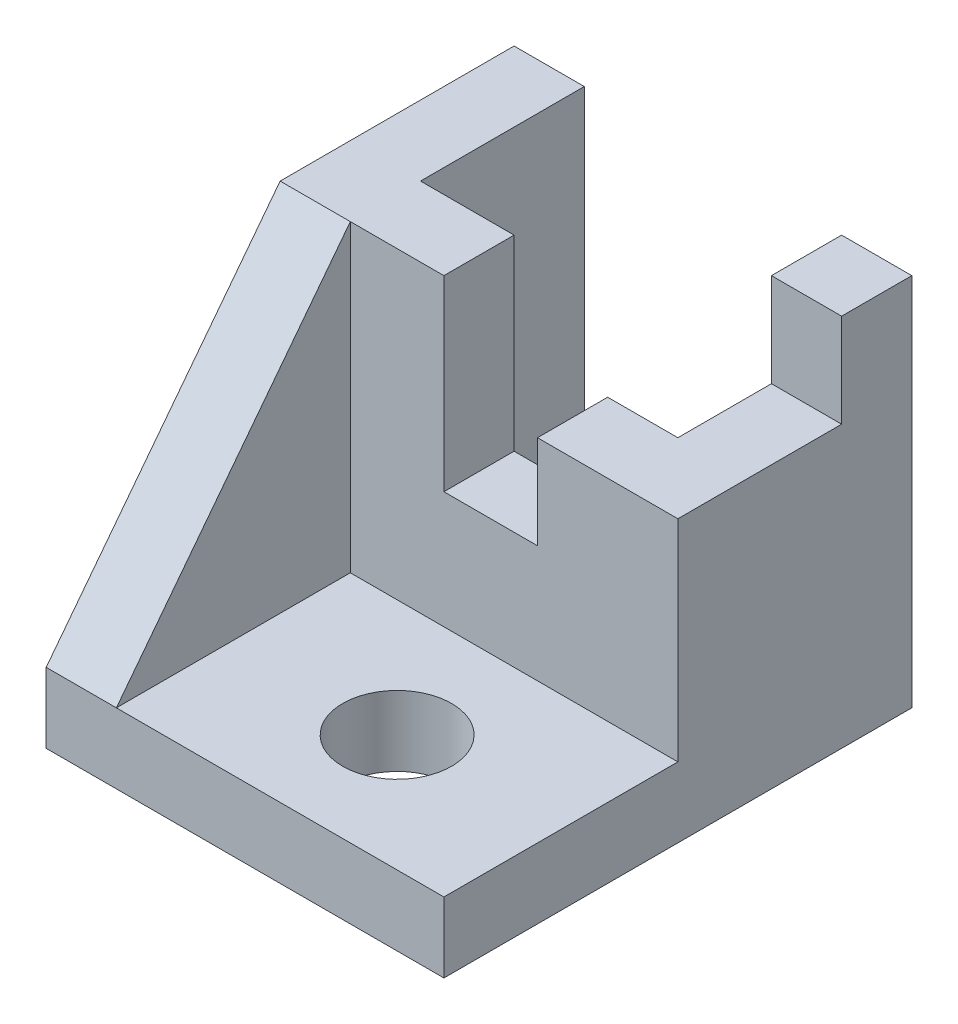
ISO-10303-21;
HEADER;
FILE_DESCRIPTION(('STEP AP214'),'2;1');
FILE_NAME('part.step','',(''),(''),'','','');
FILE_SCHEMA(('AUTOMOTIVE_DESIGN { 1 0 10303 214 1 1 1 1 }'));
ENDSEC;
DATA;
#1=APPLICATION_CONTEXT('core data for automotive mechanical design processes');
#2=APPLICATION_PROTOCOL_DEFINITION('international standard','automotive_design',2000,#1);
#3=PRODUCT_CONTEXT('',#1,'mechanical');
#4=PRODUCT('Part','Part','',(#3));
#5=PRODUCT_RELATED_PRODUCT_CATEGORY('part','',(#4));
#6=PRODUCT_DEFINITION_FORMATION('','',#4);
#7=PRODUCT_DEFINITION_CONTEXT('part definition',#1,'design');
#8=PRODUCT_DEFINITION('design','',#6,#7);
#9=PRODUCT_DEFINITION_SHAPE('','',#8);
#10=(LENGTH_UNIT() NAMED_UNIT(*) SI_UNIT(.MILLI.,.METRE.));
#11=(NAMED_UNIT(*) PLANE_ANGLE_UNIT() SI_UNIT($,.RADIAN.));
#12=(NAMED_UNIT(*) SI_UNIT($,.STERADIAN.) SOLID_ANGLE_UNIT());
#13=UNCERTAINTY_MEASURE_WITH_UNIT(LENGTH_MEASURE(1.E-05),#10,'distance_accuracy_value','');
#14=(GEOMETRIC_REPRESENTATION_CONTEXT(3) GLOBAL_UNCERTAINTY_ASSIGNED_CONTEXT((#13)) GLOBAL_UNIT_ASSIGNED_CONTEXT((#10,
#11,#12)) REPRESENTATION_CONTEXT('',''));
#15=CARTESIAN_POINT('',(0.,0.,0.));
#16=DIRECTION('',(0.,0.,1.));
#17=DIRECTION('',(1.,0.,0.));
#18=AXIS2_PLACEMENT_3D('',#15,#16,#17);
#19=CARTESIAN_POINT('',(0.,15.,0.));
#20=DIRECTION('',(0.,-1.,0.));
#21=DIRECTION('',(0.,0.,-1.));
#22=AXIS2_PLACEMENT_3D('',#19,#20,#21);
#23=PLANE('',#22);
#24=DIRECTION('',(-1.,0.,0.));
#25=VECTOR('',#24,1.);
#26=CARTESIAN_POINT('',(0.,15.,-15.));
#27=LINE('',#26,#25);
#28=CARTESIAN_POINT('',(27.5,15.,-15.));
#29=VERTEX_POINT('',#28);
#30=CARTESIAN_POINT('',(-27.5,15.,-15.));
#31=VERTEX_POINT('',#30);
#32=EDGE_CURVE('E158',#29,#31,#27,.T.);
#33=ORIENTED_EDGE('',*,*,#32,.F.);
#34=DIRECTION('',(0.,0.,1.));
#35=VECTOR('',#34,1.);
#36=CARTESIAN_POINT('',(27.5,15.,0.));
#37=LINE('',#36,#35);
#38=CARTESIAN_POINT('',(27.5,15.,-50.));
#39=VERTEX_POINT('',#38);
#40=EDGE_CURVE('E161',#39,#29,#37,.T.);
#41=ORIENTED_EDGE('',*,*,#40,.F.);
#42=DIRECTION('',(-1.,0.,0.));
#43=VECTOR('',#42,1.);
#44=CARTESIAN_POINT('',(-42.5,15.,-50.));
#45=LINE('',#44,#43);
#46=CARTESIAN_POINT('',(-27.5,15.,-50.));
#47=VERTEX_POINT('',#46);
#48=EDGE_CURVE('E227',#39,#47,#45,.T.);
#49=ORIENTED_EDGE('',*,*,#48,.T.);
#50=DIRECTION('',(0.,0.,1.));
#51=VECTOR('',#50,1.);
#52=CARTESIAN_POINT('',(-27.5,15.,0.));
#53=LINE('',#52,#51);
#54=EDGE_CURVE('E168',#47,#31,#53,.T.);
#55=ORIENTED_EDGE('',*,*,#54,.T.);
#56=EDGE_LOOP('',(#33,#41,#49,#55));
#57=FACE_BOUND('',#56,.T.);
#58=ADVANCED_FACE('F41',(#57),#23,.F.);
#59=CARTESIAN_POINT('',(27.5,0.,0.));
#60=DIRECTION('',(1.,0.,0.));
#61=DIRECTION('',(0.,0.,-1.));
#62=AXIS2_PLACEMENT_3D('',#59,#60,#61);
#63=PLANE('',#62);
#64=DIRECTION('',(0.,1.,0.));
#65=VECTOR('',#64,1.);
#66=CARTESIAN_POINT('',(27.5,60.,-15.));
#67=LINE('',#66,#65);
#68=CARTESIAN_POINT('',(27.5,60.,-15.));
#69=VERTEX_POINT('',#68);
#70=EDGE_CURVE('E171',#29,#69,#67,.T.);
#71=ORIENTED_EDGE('',*,*,#70,.T.);
#72=DIRECTION('',(0.,0.,1.));
#73=VECTOR('',#72,1.);
#74=CARTESIAN_POINT('',(27.5,60.,0.));
#75=LINE('',#74,#73);
#76=CARTESIAN_POINT('',(27.5,60.,-35.));
#77=VERTEX_POINT('',#76);
#78=EDGE_CURVE('E190',#77,#69,#75,.T.);
#79=ORIENTED_EDGE('',*,*,#78,.F.);
#80=DIRECTION('',(0.,-1.,0.));
#81=VECTOR('',#80,1.);
#82=CARTESIAN_POINT('',(27.5,0.,-35.));
#83=LINE('',#82,#81);
#84=CARTESIAN_POINT('',(27.5,80.,-35.));
#85=VERTEX_POINT('',#84);
#86=EDGE_CURVE('E200',#85,#77,#83,.T.);
#87=ORIENTED_EDGE('',*,*,#86,.F.);
#88=DIRECTION('',(0.,0.,1.));
#89=VECTOR('',#88,1.);
#90=CARTESIAN_POINT('',(27.5,80.,0.));
#91=LINE('',#90,#89);
#92=CARTESIAN_POINT('',(27.5,80.,-50.));
#93=VERTEX_POINT('',#92);
#94=EDGE_CURVE('E186',#93,#85,#91,.T.);
#95=ORIENTED_EDGE('',*,*,#94,.F.);
#96=DIRECTION('',(0.,1.,0.));
#97=VECTOR('',#96,1.);
#98=CARTESIAN_POINT('',(27.5,0.,-50.));
#99=LINE('',#98,#97);
#100=EDGE_CURVE('E187',#39,#93,#99,.T.);
#101=ORIENTED_EDGE('',*,*,#100,.F.);
#102=ORIENTED_EDGE('',*,*,#40,.T.);
#103=EDGE_LOOP('',(#71,#79,#87,#95,#101,#102));
#104=FACE_BOUND('',#103,.T.);
#105=ADVANCED_FACE('F182',(#104),#63,.F.);
#106=CARTESIAN_POINT('',(-27.5,0.,0.));
#107=DIRECTION('',(1.,0.,0.));
#108=DIRECTION('',(0.,0.,-1.));
#109=AXIS2_PLACEMENT_3D('',#106,#107,#108);
#110=PLANE('',#109);
#111=DIRECTION('',(0.,1.,0.));
#112=VECTOR('',#111,1.);
#113=CARTESIAN_POINT('',(-27.5,20.,-15.));
#114=LINE('',#113,#112);
#115=CARTESIAN_POINT('',(-27.5,80.,-15.));
#116=VERTEX_POINT('',#115);
#117=EDGE_CURVE('E57',#31,#116,#114,.T.);
#118=ORIENTED_EDGE('',*,*,#117,.F.);
#119=ORIENTED_EDGE('',*,*,#54,.F.);
#120=DIRECTION('',(0.,-1.,0.));
#121=VECTOR('',#120,1.);
#122=CARTESIAN_POINT('',(-27.5,15.,-50.));
#123=LINE('',#122,#121);
#124=CARTESIAN_POINT('',(-27.5,80.,-50.));
#125=VERTEX_POINT('',#124);
#126=EDGE_CURVE('E283',#125,#47,#123,.T.);
#127=ORIENTED_EDGE('',*,*,#126,.F.);
#128=DIRECTION('',(0.,0.,-1.));
#129=VECTOR('',#128,1.);
#130=CARTESIAN_POINT('',(-27.5,80.,-50.));
#131=LINE('',#130,#129);
#132=EDGE_CURVE('E287',#116,#125,#131,.T.);
#133=ORIENTED_EDGE('',*,*,#132,.F.);
#134=EDGE_LOOP('',(#118,#119,#127,#133));
#135=FACE_BOUND('',#134,.T.);
#136=ADVANCED_FACE('F341',(#135),#110,.T.);
#137=CARTESIAN_POINT('',(7.50000000000001,15.,25.));
#138=DIRECTION('',(0.,1.,0.));
#139=DIRECTION('',(0.,0.,1.));
#140=AXIS2_PLACEMENT_3D('',#137,#138,#139);
#141=CIRCLE('',#140,11.6364230481532);
#142=CARTESIAN_POINT('',(7.50000000000001,15.,36.6364230481532));
#143=VERTEX_POINT('',#142);
#144=EDGE_CURVE('E328',#143,#143,#141,.T.);
#145=ORIENTED_EDGE('',*,*,#144,.F.);
#146=EDGE_LOOP('',(#145));
#147=FACE_BOUND('',#146,.T.);
#148=DIRECTION('',(1.,0.,0.));
#149=VECTOR('',#148,1.);
#150=CARTESIAN_POINT('',(27.5,15.,0.));
#151=LINE('',#150,#149);
#152=CARTESIAN_POINT('',(-27.5,15.,0.));
#153=VERTEX_POINT('',#152);
#154=CARTESIAN_POINT('',(42.5,15.,0.));
#155=VERTEX_POINT('',#154);
#156=EDGE_CURVE('E222',#153,#155,#151,.T.);
#157=ORIENTED_EDGE('',*,*,#156,.F.);
#158=CARTESIAN_POINT('',(-27.5,15.,50.));
#159=VERTEX_POINT('',#158);
#160=EDGE_CURVE('E61',#153,#159,#53,.T.);
#161=ORIENTED_EDGE('',*,*,#160,.T.);
#162=DIRECTION('',(1.,0.,0.));
#163=VECTOR('',#162,1.);
#164=CARTESIAN_POINT('',(-42.5,15.,50.));
#165=LINE('',#164,#163);
#166=CARTESIAN_POINT('',(42.5,15.,50.));
#167=VERTEX_POINT('',#166);
#168=EDGE_CURVE('E229',#159,#167,#165,.T.);
#169=ORIENTED_EDGE('',*,*,#168,.T.);
#170=DIRECTION('',(0.,0.,-1.));
#171=VECTOR('',#170,1.);
#172=CARTESIAN_POINT('',(42.5,15.,50.));
#173=LINE('',#172,#171);
#174=EDGE_CURVE('E223',#167,#155,#173,.T.);
#175=ORIENTED_EDGE('',*,*,#174,.T.);
#176=EDGE_LOOP('',(#157,#161,#169,#175));
#177=FACE_BOUND('',#176,.T.);
#178=ADVANCED_FACE('F270',(#147,#177),#23,.F.);
#179=CARTESIAN_POINT('',(42.5,15.,50.));
#180=DIRECTION('',(-1.,0.,0.));
#181=DIRECTION('',(0.,0.,1.));
#182=AXIS2_PLACEMENT_3D('',#179,#180,#181);
#183=PLANE('',#182);
#184=DIRECTION('',(0.,0.,-1.));
#185=VECTOR('',#184,1.);
#186=CARTESIAN_POINT('',(42.5,0.,50.));
#187=LINE('',#186,#185);
#188=CARTESIAN_POINT('',(42.5,0.,50.));
#189=VERTEX_POINT('',#188);
#190=CARTESIAN_POINT('',(42.5,0.,-50.));
#191=VERTEX_POINT('',#190);
#192=EDGE_CURVE('E213',#189,#191,#187,.T.);
#193=ORIENTED_EDGE('',*,*,#192,.T.);
#194=DIRECTION('',(0.,-1.,0.));
#195=VECTOR('',#194,1.);
#196=CARTESIAN_POINT('',(42.5,15.,-50.));
#197=LINE('',#196,#195);
#198=CARTESIAN_POINT('',(42.5,80.,-50.));
#199=VERTEX_POINT('',#198);
#200=EDGE_CURVE('E11',#199,#191,#197,.T.);
#201=ORIENTED_EDGE('',*,*,#200,.F.);
#202=DIRECTION('',(0.,0.,1.));
#203=VECTOR('',#202,1.);
#204=CARTESIAN_POINT('',(42.5,80.,0.));
#205=LINE('',#204,#203);
#206=CARTESIAN_POINT('',(42.5,80.,-35.));
#207=VERTEX_POINT('',#206);
#208=EDGE_CURVE('E206',#199,#207,#205,.T.);
#209=ORIENTED_EDGE('',*,*,#208,.T.);
#210=DIRECTION('',(0.,-1.,0.));
#211=VECTOR('',#210,1.);
#212=CARTESIAN_POINT('',(42.5,0.,-35.));
#213=LINE('',#212,#211);
#214=CARTESIAN_POINT('',(42.5,60.,-35.));
#215=VERTEX_POINT('',#214);
#216=EDGE_CURVE('E192',#207,#215,#213,.T.);
#217=ORIENTED_EDGE('',*,*,#216,.T.);
#218=DIRECTION('',(0.,0.,1.));
#219=VECTOR('',#218,1.);
#220=CARTESIAN_POINT('',(42.5,60.,0.));
#221=LINE('',#220,#219);
#222=CARTESIAN_POINT('',(42.5,60.,0.));
#223=VERTEX_POINT('',#222);
#224=EDGE_CURVE('E202',#215,#223,#221,.T.);
#225=ORIENTED_EDGE('',*,*,#224,.T.);
#226=DIRECTION('',(0.,-1.,0.));
#227=VECTOR('',#226,1.);
#228=CARTESIAN_POINT('',(42.5,0.,0.));
#229=LINE('',#228,#227);
#230=EDGE_CURVE('E201',#223,#155,#229,.T.);
#231=ORIENTED_EDGE('',*,*,#230,.T.);
#232=ORIENTED_EDGE('',*,*,#174,.F.);
#233=DIRECTION('',(0.,-1.,0.));
#234=VECTOR('',#233,1.);
#235=CARTESIAN_POINT('',(42.5,15.,50.));
#236=LINE('',#235,#234);
#237=EDGE_CURVE('E234',#167,#189,#236,.T.);
#238=ORIENTED_EDGE('',*,*,#237,.T.);
#239=EDGE_LOOP('',(#193,#201,#209,#217,#225,#231,#232,#238));
#240=FACE_BOUND('',#239,.T.);
#241=ADVANCED_FACE('F43',(#240),#183,.F.);
#242=CARTESIAN_POINT('',(-42.5,15.,-50.));
#243=DIRECTION('',(0.,0.,1.));
#244=DIRECTION('',(1.,0.,0.));
#245=AXIS2_PLACEMENT_3D('',#242,#243,#244);
#246=PLANE('',#245);
#247=DIRECTION('',(-1.,0.,0.));
#248=VECTOR('',#247,1.);
#249=CARTESIAN_POINT('',(-42.5,0.,-50.));
#250=LINE('',#249,#248);
#251=CARTESIAN_POINT('',(-42.5,0.,-50.));
#252=VERTEX_POINT('',#251);
#253=EDGE_CURVE('E240',#191,#252,#250,.T.);
#254=ORIENTED_EDGE('',*,*,#253,.T.);
#255=DIRECTION('',(0.,-1.,0.));
#256=VECTOR('',#255,1.);
#257=CARTESIAN_POINT('',(-42.5,15.,-50.));
#258=LINE('',#257,#256);
#259=CARTESIAN_POINT('',(-42.5,80.,-50.));
#260=VERTEX_POINT('',#259);
#261=EDGE_CURVE('E47',#260,#252,#258,.T.);
#262=ORIENTED_EDGE('',*,*,#261,.F.);
#263=DIRECTION('',(-1.,0.,0.));
#264=VECTOR('',#263,1.);
#265=CARTESIAN_POINT('',(-27.5,80.,-50.));
#266=LINE('',#265,#264);
#267=EDGE_CURVE('E203',#125,#260,#266,.T.);
#268=ORIENTED_EDGE('',*,*,#267,.F.);
#269=ORIENTED_EDGE('',*,*,#126,.T.);
#270=ORIENTED_EDGE('',*,*,#48,.F.);
#271=ORIENTED_EDGE('',*,*,#100,.T.);
#272=DIRECTION('',(1.,0.,0.));
#273=VECTOR('',#272,1.);
#274=CARTESIAN_POINT('',(27.5,80.,-50.));
#275=LINE('',#274,#273);
#276=EDGE_CURVE('E217',#93,#199,#275,.T.);
#277=ORIENTED_EDGE('',*,*,#276,.T.);
#278=ORIENTED_EDGE('',*,*,#200,.T.);
#279=EDGE_LOOP('',(#254,#262,#268,#269,#270,#271,#277,#278));
#280=FACE_BOUND('',#279,.T.);
#281=ADVANCED_FACE('F352',(#280),#246,.F.);
#282=CARTESIAN_POINT('',(-42.5,15.,50.));
#283=DIRECTION('',(1.,0.,0.));
#284=DIRECTION('',(0.,0.,-1.));
#285=AXIS2_PLACEMENT_3D('',#282,#283,#284);
#286=PLANE('',#285);
#287=DIRECTION('',(0.,-1.,0.));
#288=VECTOR('',#287,1.);
#289=CARTESIAN_POINT('',(-42.5,15.,50.));
#290=LINE('',#289,#288);
#291=CARTESIAN_POINT('',(-42.5,15.,50.));
#292=VERTEX_POINT('',#291);
#293=CARTESIAN_POINT('',(-42.5,0.,50.));
#294=VERTEX_POINT('',#293);
#295=EDGE_CURVE('E242',#292,#294,#290,.T.);
#296=ORIENTED_EDGE('',*,*,#295,.F.);
#297=DIRECTION('',(0.,0.7926239891046,-0.609710760849692));
#298=VECTOR('',#297,1.);
#299=CARTESIAN_POINT('',(-42.5,80.,0.));
#300=LINE('',#299,#298);
#301=CARTESIAN_POINT('',(-42.5,80.,0.));
#302=VERTEX_POINT('',#301);
#303=EDGE_CURVE('E296',#292,#302,#300,.T.);
#304=ORIENTED_EDGE('',*,*,#303,.T.);
#305=DIRECTION('',(0.,0.,-1.));
#306=VECTOR('',#305,1.);
#307=CARTESIAN_POINT('',(-42.5,80.,-50.));
#308=LINE('',#307,#306);
#309=EDGE_CURVE('E255',#302,#260,#308,.T.);
#310=ORIENTED_EDGE('',*,*,#309,.T.);
#311=ORIENTED_EDGE('',*,*,#261,.T.);
#312=DIRECTION('',(0.,0.,1.));
#313=VECTOR('',#312,1.);
#314=CARTESIAN_POINT('',(-42.5,0.,50.));
#315=LINE('',#314,#313);
#316=EDGE_CURVE('E237',#252,#294,#315,.T.);
#317=ORIENTED_EDGE('',*,*,#316,.T.);
#318=EDGE_LOOP('',(#296,#304,#310,#311,#317));
#319=FACE_BOUND('',#318,.T.);
#320=ADVANCED_FACE('F249',(#319),#286,.F.);
#321=CARTESIAN_POINT('',(-42.5,15.,50.));
#322=DIRECTION('',(0.,0.,-1.));
#323=DIRECTION('',(-1.,0.,0.));
#324=AXIS2_PLACEMENT_3D('',#321,#322,#323);
#325=PLANE('',#324);
#326=DIRECTION('',(1.,0.,0.));
#327=VECTOR('',#326,1.);
#328=CARTESIAN_POINT('',(-42.5,0.,50.));
#329=LINE('',#328,#327);
#330=EDGE_CURVE('E226',#294,#189,#329,.T.);
#331=ORIENTED_EDGE('',*,*,#330,.T.);
#332=ORIENTED_EDGE('',*,*,#237,.F.);
#333=ORIENTED_EDGE('',*,*,#168,.F.);
#334=EDGE_CURVE('E233',#292,#159,#165,.T.);
#335=ORIENTED_EDGE('',*,*,#334,.F.);
#336=ORIENTED_EDGE('',*,*,#295,.T.);
#337=EDGE_LOOP('',(#331,#332,#333,#335,#336));
#338=FACE_BOUND('',#337,.T.);
#339=ADVANCED_FACE('F265',(#338),#325,.F.);
#340=CARTESIAN_POINT('',(0.,0.,0.));
#341=DIRECTION('',(0.,-1.,0.));
#342=DIRECTION('',(0.,0.,-1.));
#343=AXIS2_PLACEMENT_3D('',#340,#341,#342);
#344=PLANE('',#343);
#345=CARTESIAN_POINT('',(7.50000000000001,0.,25.));
#346=DIRECTION('',(0.,1.,0.));
#347=DIRECTION('',(0.,0.,1.));
#348=AXIS2_PLACEMENT_3D('',#345,#346,#347);
#349=CIRCLE('',#348,11.6364230481532);
#350=CARTESIAN_POINT('',(7.50000000000001,0.,36.6364230481532));
#351=VERTEX_POINT('',#350);
#352=EDGE_CURVE('E324',#351,#351,#349,.T.);
#353=ORIENTED_EDGE('',*,*,#352,.T.);
#354=EDGE_LOOP('',(#353));
#355=FACE_BOUND('',#354,.T.);
#356=ORIENTED_EDGE('',*,*,#192,.F.);
#357=ORIENTED_EDGE('',*,*,#330,.F.);
#358=ORIENTED_EDGE('',*,*,#316,.F.);
#359=ORIENTED_EDGE('',*,*,#253,.F.);
#360=EDGE_LOOP('',(#356,#357,#358,#359));
#361=FACE_BOUND('',#360,.T.);
#362=ADVANCED_FACE('F256',(#355,#361),#344,.T.);
#363=CARTESIAN_POINT('',(27.5,60.,0.));
#364=DIRECTION('',(0.,1.,0.));
#365=DIRECTION('',(0.,0.,1.));
#366=AXIS2_PLACEMENT_3D('',#363,#364,#365);
#367=PLANE('',#366);
#368=ORIENTED_EDGE('',*,*,#224,.F.);
#369=DIRECTION('',(1.,0.,0.));
#370=VECTOR('',#369,1.);
#371=CARTESIAN_POINT('',(27.5,60.,-35.));
#372=LINE('',#371,#370);
#373=EDGE_CURVE('E214',#77,#215,#372,.T.);
#374=ORIENTED_EDGE('',*,*,#373,.F.);
#375=ORIENTED_EDGE('',*,*,#78,.T.);
#376=DIRECTION('',(-1.,0.,0.));
#377=VECTOR('',#376,1.);
#378=CARTESIAN_POINT('',(12.5,60.,-15.));
#379=LINE('',#378,#377);
#380=CARTESIAN_POINT('',(12.5,60.,-15.));
#381=VERTEX_POINT('',#380);
#382=EDGE_CURVE('E176',#69,#381,#379,.T.);
#383=ORIENTED_EDGE('',*,*,#382,.T.);
#384=DIRECTION('',(0.,0.,1.));
#385=VECTOR('',#384,1.);
#386=CARTESIAN_POINT('',(12.5,60.,-15.));
#387=LINE('',#386,#385);
#388=CARTESIAN_POINT('',(12.5,60.,0.));
#389=VERTEX_POINT('',#388);
#390=EDGE_CURVE('E315',#381,#389,#387,.T.);
#391=ORIENTED_EDGE('',*,*,#390,.T.);
#392=DIRECTION('',(1.,0.,0.));
#393=VECTOR('',#392,1.);
#394=CARTESIAN_POINT('',(27.5,60.,0.));
#395=LINE('',#394,#393);
#396=EDGE_CURVE('E199',#389,#223,#395,.T.);
#397=ORIENTED_EDGE('',*,*,#396,.T.);
#398=EDGE_LOOP('',(#368,#374,#375,#383,#391,#397));
#399=FACE_BOUND('',#398,.T.);
#400=ADVANCED_FACE('F375',(#399),#367,.T.);
#401=CARTESIAN_POINT('',(27.5,0.,-35.));
#402=DIRECTION('',(0.,0.,1.));
#403=DIRECTION('',(0.,-1.,0.));
#404=AXIS2_PLACEMENT_3D('',#401,#402,#403);
#405=PLANE('',#404);
#406=ORIENTED_EDGE('',*,*,#216,.F.);
#407=DIRECTION('',(1.,0.,0.));
#408=VECTOR('',#407,1.);
#409=CARTESIAN_POINT('',(27.5,80.,-35.));
#410=LINE('',#409,#408);
#411=EDGE_CURVE('E216',#85,#207,#410,.T.);
#412=ORIENTED_EDGE('',*,*,#411,.F.);
#413=ORIENTED_EDGE('',*,*,#86,.T.);
#414=ORIENTED_EDGE('',*,*,#373,.T.);
#415=EDGE_LOOP('',(#406,#412,#413,#414));
#416=FACE_BOUND('',#415,.T.);
#417=ADVANCED_FACE('F368',(#416),#405,.T.);
#418=CARTESIAN_POINT('',(27.5,80.,0.));
#419=DIRECTION('',(0.,1.,0.));
#420=DIRECTION('',(0.,0.,1.));
#421=AXIS2_PLACEMENT_3D('',#418,#419,#420);
#422=PLANE('',#421);
#423=ORIENTED_EDGE('',*,*,#208,.F.);
#424=ORIENTED_EDGE('',*,*,#276,.F.);
#425=ORIENTED_EDGE('',*,*,#94,.T.);
#426=ORIENTED_EDGE('',*,*,#411,.T.);
#427=EDGE_LOOP('',(#423,#424,#425,#426));
#428=FACE_BOUND('',#427,.T.);
#429=ADVANCED_FACE('F371',(#428),#422,.T.);
#430=CARTESIAN_POINT('',(27.5,0.,0.));
#431=DIRECTION('',(0.,0.,1.));
#432=DIRECTION('',(0.,-1.,0.));
#433=AXIS2_PLACEMENT_3D('',#430,#431,#432);
#434=PLANE('',#433);
#435=ORIENTED_EDGE('',*,*,#230,.F.);
#436=ORIENTED_EDGE('',*,*,#396,.F.);
#437=DIRECTION('',(0.,-1.,0.));
#438=VECTOR('',#437,1.);
#439=CARTESIAN_POINT('',(12.5,40.,0.));
#440=LINE('',#439,#438);
#441=CARTESIAN_POINT('',(12.5,40.,0.));
#442=VERTEX_POINT('',#441);
#443=EDGE_CURVE('E318',#389,#442,#440,.T.);
#444=ORIENTED_EDGE('',*,*,#443,.T.);
#445=DIRECTION('',(-1.,0.,0.));
#446=VECTOR('',#445,1.);
#447=CARTESIAN_POINT('',(-7.49999999999999,40.,0.));
#448=LINE('',#447,#446);
#449=CARTESIAN_POINT('',(-7.49999999999999,40.,0.));
#450=VERTEX_POINT('',#449);
#451=EDGE_CURVE('E179',#442,#450,#448,.T.);
#452=ORIENTED_EDGE('',*,*,#451,.T.);
#453=DIRECTION('',(0.,1.,0.));
#454=VECTOR('',#453,1.);
#455=CARTESIAN_POINT('',(-7.49999999999999,20.,0.));
#456=LINE('',#455,#454);
#457=CARTESIAN_POINT('',(-7.49999999999999,80.,0.));
#458=VERTEX_POINT('',#457);
#459=EDGE_CURVE('E279',#450,#458,#456,.T.);
#460=ORIENTED_EDGE('',*,*,#459,.T.);
#461=DIRECTION('',(1.,0.,0.));
#462=VECTOR('',#461,1.);
#463=CARTESIAN_POINT('',(-27.5,80.,0.));
#464=LINE('',#463,#462);
#465=CARTESIAN_POINT('',(-27.5,80.,0.));
#466=VERTEX_POINT('',#465);
#467=EDGE_CURVE('E274',#466,#458,#464,.T.);
#468=ORIENTED_EDGE('',*,*,#467,.F.);
#469=DIRECTION('',(0.,1.,0.));
#470=VECTOR('',#469,1.);
#471=CARTESIAN_POINT('',(-27.5,20.,0.));
#472=LINE('',#471,#470);
#473=EDGE_CURVE('E275',#153,#466,#472,.T.);
#474=ORIENTED_EDGE('',*,*,#473,.F.);
#475=ORIENTED_EDGE('',*,*,#156,.T.);
#476=EDGE_LOOP('',(#435,#436,#444,#452,#460,#468,#474,#475));
#477=FACE_BOUND('',#476,.T.);
#478=ADVANCED_FACE('F268',(#477),#434,.T.);
#479=CARTESIAN_POINT('',(-27.5,80.,-50.));
#480=DIRECTION('',(0.,1.,0.));
#481=DIRECTION('',(0.,0.,1.));
#482=AXIS2_PLACEMENT_3D('',#479,#480,#481);
#483=PLANE('',#482);
#484=ORIENTED_EDGE('',*,*,#309,.F.);
#485=DIRECTION('',(-1.,0.,0.));
#486=VECTOR('',#485,1.);
#487=CARTESIAN_POINT('',(-27.5,80.,0.));
#488=LINE('',#487,#486);
#489=EDGE_CURVE('E292',#466,#302,#488,.T.);
#490=ORIENTED_EDGE('',*,*,#489,.F.);
#491=ORIENTED_EDGE('',*,*,#467,.T.);
#492=DIRECTION('',(0.,0.,-1.));
#493=VECTOR('',#492,1.);
#494=CARTESIAN_POINT('',(-7.49999999999999,80.,0.));
#495=LINE('',#494,#493);
#496=CARTESIAN_POINT('',(-7.49999999999999,80.,-15.));
#497=VERTEX_POINT('',#496);
#498=EDGE_CURVE('E310',#458,#497,#495,.T.);
#499=ORIENTED_EDGE('',*,*,#498,.T.);
#500=DIRECTION('',(-1.,0.,0.));
#501=VECTOR('',#500,1.);
#502=CARTESIAN_POINT('',(-7.49999999999999,80.,-15.));
#503=LINE('',#502,#501);
#504=EDGE_CURVE('E276',#497,#116,#503,.T.);
#505=ORIENTED_EDGE('',*,*,#504,.T.);
#506=ORIENTED_EDGE('',*,*,#132,.T.);
#507=ORIENTED_EDGE('',*,*,#267,.T.);
#508=EDGE_LOOP('',(#484,#490,#491,#499,#505,#506,#507));
#509=FACE_BOUND('',#508,.T.);
#510=ADVANCED_FACE('F370',(#509),#483,.T.);
#511=ORIENTED_EDGE('',*,*,#160,.F.);
#512=ORIENTED_EDGE('',*,*,#473,.T.);
#513=DIRECTION('',(0.,0.7926239891046,-0.609710760849692));
#514=VECTOR('',#513,1.);
#515=CARTESIAN_POINT('',(-27.5,80.,0.));
#516=LINE('',#515,#514);
#517=EDGE_CURVE('E282',#159,#466,#516,.T.);
#518=ORIENTED_EDGE('',*,*,#517,.F.);
#519=EDGE_LOOP('',(#511,#512,#518));
#520=FACE_BOUND('',#519,.T.);
#521=ADVANCED_FACE('F281',(#520),#110,.T.);
#522=CARTESIAN_POINT('',(-27.5,80.,0.));
#523=DIRECTION('',(0.,0.609710760849692,0.7926239891046));
#524=DIRECTION('',(0.,-0.7926239891046,0.609710760849693));
#525=AXIS2_PLACEMENT_3D('',#522,#523,#524);
#526=PLANE('',#525);
#527=ORIENTED_EDGE('',*,*,#303,.F.);
#528=ORIENTED_EDGE('',*,*,#334,.T.);
#529=ORIENTED_EDGE('',*,*,#517,.T.);
#530=ORIENTED_EDGE('',*,*,#489,.T.);
#531=EDGE_LOOP('',(#527,#528,#529,#530));
#532=FACE_BOUND('',#531,.T.);
#533=ADVANCED_FACE('F300',(#532),#526,.T.);
#534=CARTESIAN_POINT('',(-7.49999999999999,20.,-15.));
#535=DIRECTION('',(0.,0.,-1.));
#536=DIRECTION('',(-1.,0.,0.));
#537=AXIS2_PLACEMENT_3D('',#534,#535,#536);
#538=PLANE('',#537);
#539=DIRECTION('',(0.,1.,0.));
#540=VECTOR('',#539,1.);
#541=CARTESIAN_POINT('',(-7.49999999999999,20.,-15.));
#542=LINE('',#541,#540);
#543=CARTESIAN_POINT('',(-7.49999999999998,40.,-15.));
#544=VERTEX_POINT('',#543);
#545=EDGE_CURVE('E301',#544,#497,#542,.T.);
#546=ORIENTED_EDGE('',*,*,#545,.F.);
#547=DIRECTION('',(-1.,0.,0.));
#548=VECTOR('',#547,1.);
#549=CARTESIAN_POINT('',(12.5,40.,-15.));
#550=LINE('',#549,#548);
#551=CARTESIAN_POINT('',(12.5,40.,-15.));
#552=VERTEX_POINT('',#551);
#553=EDGE_CURVE('E314',#552,#544,#550,.T.);
#554=ORIENTED_EDGE('',*,*,#553,.F.);
#555=DIRECTION('',(0.,-1.,0.));
#556=VECTOR('',#555,1.);
#557=CARTESIAN_POINT('',(12.5,40.,-15.));
#558=LINE('',#557,#556);
#559=EDGE_CURVE('E323',#381,#552,#558,.T.);
#560=ORIENTED_EDGE('',*,*,#559,.F.);
#561=ORIENTED_EDGE('',*,*,#382,.F.);
#562=ORIENTED_EDGE('',*,*,#70,.F.);
#563=ORIENTED_EDGE('',*,*,#32,.T.);
#564=ORIENTED_EDGE('',*,*,#117,.T.);
#565=ORIENTED_EDGE('',*,*,#504,.F.);
#566=EDGE_LOOP('',(#546,#554,#560,#561,#562,#563,#564,#565));
#567=FACE_BOUND('',#566,.T.);
#568=ADVANCED_FACE('F173',(#567),#538,.T.);
#569=CARTESIAN_POINT('',(-7.49999999999999,20.,0.));
#570=DIRECTION('',(1.,0.,0.));
#571=DIRECTION('',(0.,0.,-1.));
#572=AXIS2_PLACEMENT_3D('',#569,#570,#571);
#573=PLANE('',#572);
#574=DIRECTION('',(0.,0.,1.));
#575=VECTOR('',#574,1.);
#576=CARTESIAN_POINT('',(-7.49999999999999,40.,0.));
#577=LINE('',#576,#575);
#578=EDGE_CURVE('E170',#544,#450,#577,.T.);
#579=ORIENTED_EDGE('',*,*,#578,.F.);
#580=ORIENTED_EDGE('',*,*,#545,.T.);
#581=ORIENTED_EDGE('',*,*,#498,.F.);
#582=ORIENTED_EDGE('',*,*,#459,.F.);
#583=EDGE_LOOP('',(#579,#580,#581,#582));
#584=FACE_BOUND('',#583,.T.);
#585=ADVANCED_FACE('F392',(#584),#573,.T.);
#586=CARTESIAN_POINT('',(-7.49999999999999,40.,-15.));
#587=DIRECTION('',(0.,1.,0.));
#588=DIRECTION('',(0.,0.,1.));
#589=AXIS2_PLACEMENT_3D('',#586,#587,#588);
#590=PLANE('',#589);
#591=ORIENTED_EDGE('',*,*,#553,.T.);
#592=ORIENTED_EDGE('',*,*,#578,.T.);
#593=ORIENTED_EDGE('',*,*,#451,.F.);
#594=DIRECTION('',(0.,0.,1.));
#595=VECTOR('',#594,1.);
#596=CARTESIAN_POINT('',(12.5,40.,-15.));
#597=LINE('',#596,#595);
#598=EDGE_CURVE('E166',#552,#442,#597,.T.);
#599=ORIENTED_EDGE('',*,*,#598,.F.);
#600=EDGE_LOOP('',(#591,#592,#593,#599));
#601=FACE_BOUND('',#600,.T.);
#602=ADVANCED_FACE('F407',(#601),#590,.T.);
#603=CARTESIAN_POINT('',(12.5,40.,-15.));
#604=DIRECTION('',(-1.,0.,0.));
#605=DIRECTION('',(0.,0.,1.));
#606=AXIS2_PLACEMENT_3D('',#603,#604,#605);
#607=PLANE('',#606);
#608=ORIENTED_EDGE('',*,*,#443,.F.);
#609=ORIENTED_EDGE('',*,*,#390,.F.);
#610=ORIENTED_EDGE('',*,*,#559,.T.);
#611=ORIENTED_EDGE('',*,*,#598,.T.);
#612=EDGE_LOOP('',(#608,#609,#610,#611));
#613=FACE_BOUND('',#612,.T.);
#614=ADVANCED_FACE('F339',(#613),#607,.T.);
#615=CARTESIAN_POINT('',(7.50000000000001,0.,25.));
#616=DIRECTION('',(0.,1.,0.));
#617=DIRECTION('',(0.,0.,1.));
#618=AXIS2_PLACEMENT_3D('',#615,#616,#617);
#619=CYLINDRICAL_SURFACE('',#618,11.6364230481532);
#620=ORIENTED_EDGE('',*,*,#352,.F.);
#621=EDGE_LOOP('',(#620));
#622=FACE_BOUND('',#621,.T.);
#623=ORIENTED_EDGE('',*,*,#144,.T.);
#624=EDGE_LOOP('',(#623));
#625=FACE_BOUND('',#624,.T.);
#626=ADVANCED_FACE('F337',(#622,#625),#619,.F.);
#627=CLOSED_SHELL('',(#58,#105,#136,#178,#241,#281,#320,#339,#362,#400,#417,#429,#478,#510,#521,
#533,#568,#585,#602,#614,#626));
#628=MANIFOLD_SOLID_BREP('B2',#627);
#629=ADVANCED_BREP_SHAPE_REPRESENTATION('',(#18,#628),#14);
#630=SHAPE_DEFINITION_REPRESENTATION(#9,#629);
ENDSEC;
END-ISO-10303-21;
